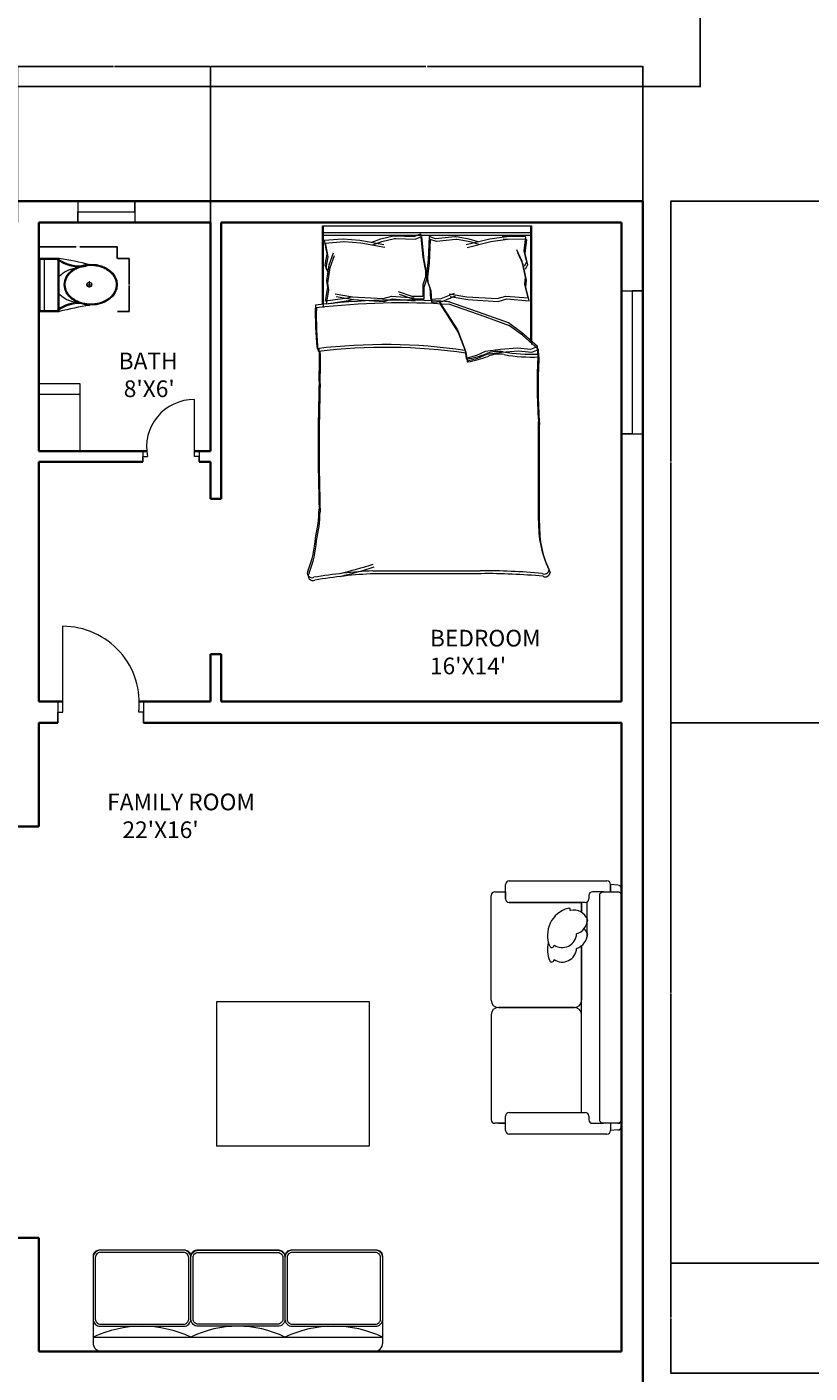
# Model space of a CAD drawing. Units: inches. Extents: x 2185 to 4426, y 1138 to 3073.
# Tile 6 of 14: x 2832 to 3160, y 1834 to 2400. Entities that reach past the tile are written whole.
import ezdxf

# ---------------------------------------------------------------- set-up
doc = ezdxf.new("R2010")
doc.units = ezdxf.units.IN
for name, color, linetype, lineweight in [('A-ANNO-DIMS', 2, 'Continuous', 18), ('A-ANNO-SYMB', 2, 'Continuous', 25), ('A-AREA-IDEN', 7, 'Continuous', 18), ('A-DOOR', 3, 'Continuous', 18), ('A-FLOR-CASE', 32, 'Continuous', 18), ('A-FLOR-FIXT', 9, 'Continuous', 18), ('A-FURN', 8, 'Continuous', 18), ('A-GLAZ', 4, 'Continuous', 18), ('A-WALL', 7, 'Continuous', 35)]:
    doc.layers.add(name, color=color, linetype=linetype, lineweight=lineweight)
doc.styles.get("Standard").update_dxf_attribs({"font": 'arial.ttf'})
doc.dimstyles.get("Standard").update_dxf_attribs({"dimtxt": 0.18, "dimasz": 0.18, "dimexe": 0.18, "dimexo": 0.0625, "dimgap": 0.09, "dimtad": 0, "dimtih": 1, "dimtoh": 1, "dimdec": 4, "dimzin": 0, "dimdsep": 46, "dimtxsty": 'Standard', "dimcen": 0.09, "dimadec": 0, "dimazin": 0, "dimtfac": 1, "dimtdec": 4, "dimtofl": 0, "dimtmove": 0, "dimatfit": 3, "dimfxl": 1, "dimtolj": 1, "dimtzin": 0, "dimarcsym": 0})

# ---------------------------------------------------------------- blocks, each defined once
blk = doc.blocks.new('A$C31115884')
for p, q in [((283, 498), (223, 498)), ((258, 466), (258, 523)), ((0, 200), (0, 0)), ((520, 200), (0, 200)), ((10, 190), (10, 10)), ((510, 190), (10, 190)), ((510, 10), (510, 190)), ((520, 0), (520, 200)), ((510, 54), (0, 54)), ((10, 10), (510, 10)), ((0, 0), (520, 0))]:
    blk.add_line(p, q)
blk.add_circle((256, 496), 23.6)
for centre, radius, start, end in [((2778, -205), 2807, 165.4549, 171.7133), ((-295, 403), 365, 324.2091, 9.3499), ((-295, 403), 375, 324.2091, 9.3499), ((139, 406), 293, 315.8436, 2.6563), ((806, 403), 375, 179.2036, 215.7909), ((806, 403), 365, 170.6501, 215.7909), ((3237, 905), 2807, 188.2867, 194.5451), ((384, 406), 293, 190.2774, 224.1564)]:
    blk.add_arc(centre, radius, start, end)
blk.add_ellipse((256, 510), major_axis=(0, -261), ratio=0.772727)
blk.add_open_spline([(256, 259), (263, 259), (270, 260), (288, 262), (299, 265), (320, 273), (330, 278), (350, 291), (360, 299), (378, 316), (386, 326), (402, 347), (409, 358), (421, 383), (427, 395), (436, 422), (440, 436), (445, 465), (447, 480), (448, 509), (448, 524), (445, 553), (443, 568), (436, 596), (432, 610), (422, 636), (416, 649), (402, 672), (395, 683), (379, 703), (370, 712), (351, 728), (341, 735), (321, 746), (310, 751), (289, 757), (278, 759), (256, 761), (245, 761), (223, 757), (212, 754), (191, 746), (181, 741), (161, 728), (151, 720), (133, 703), (125, 693), (110, 672), (103, 660), (90, 636), (85, 623), (76, 596), (72, 582), (67, 553), (66, 538), (64, 509), (65, 494), (68, 465), (70, 450), (77, 422), (81, 408), (91, 382), (97, 370), (111, 346), (118, 335), (135, 316), (144, 307), (162, 291), (172, 284), (193, 273), (203, 269), (225, 262), (236, 260), (250, 259), (253, 259), (256, 259)], degree=3, knots=[0, 0, 0, 0, 0.110105, 0.110105, 0.285049, 0.285049, 0.459994, 0.459994, 0.634938, 0.634938, 0.809882, 0.809882, 0.984827, 0.984827, 1.159771, 1.159771, 1.334715, 1.334715, 1.50966, 1.50966, 1.684604, 1.684604, 1.859549, 1.859549, 2.034493, 2.034493, 2.209437, 2.209437, 2.384382, 2.384382, 2.559326, 2.559326, 2.73427, 2.73427, 2.909215, 2.909215, 3.084159, 3.084159, 3.259103, 3.259103, 3.434048, 3.434048, 3.608992, 3.608992, 3.783936, 3.783936, 3.958881, 3.958881, 4.133825, 4.133825, 4.30877, 4.30877, 4.483714, 4.483714, 4.658658, 4.658658, 4.833603, 4.833603, 5.008547, 5.008547, 5.183491, 5.183491, 5.358436, 5.358436, 5.53338, 5.53338, 5.708324, 5.708324, 5.883269, 5.883269, 6.058213, 6.058213, 6.233158, 6.233158, 6.283185, 6.283185, 6.283185, 6.283185])
blk = doc.blocks.new('BED-DOUBLE')
for p, q in [((50.74, 96.68), (44.79, 89.9)), ((51.91, 97.09), (45.96, 90.32)), ((53.93, 96.82), (50.74, 96.68, 7.08)), ((51.87, 93.87), (50.74, 96.68)), ((55.1, 97.24), (51.91, 97.09, 7.08)), ((53.04, 94.28), (51.91, 97.09)), ((0, 93.75), (0, 94.16)), ((0, 94.16), (1.36, 94.16)), ((0, 93.75), (48.66, 93.75)), ((0, 6.35), (0, 93.75)), ((1.17, 94.16), (49.83, 94.16)), ((2.8, 6.35), (2.8, 93.75)), ((3.97, 6.77), (3.97, 94.16)), ((4.68, 91.64), (4.5, 81.76)), ((4.68, 91.64), (10.55, 90.94)), ((5.85, 92.05), (5.67, 82.18)), ((5.85, 92.05), (11.72, 91.36)), ((10.55, 90.94), (15.25, 92.03)), ((16.27, 90.59), (11.37, 88.43)), ((11.72, 91.36), (16.42, 92.45)), ((21.63, 91.64), (15.1, 90.17)), ((15.25, 92.03), (17.16, 91.09)), ((22.8, 92.05), (16.27, 90.59)), ((16.42, 92.45), (18.33, 91.51)), ((24.57, 91.29), (21.63, 91.64)), ((25.74, 91.71), (22.8, 92.05)), ((30.31, 92.71), (24.57, 91.29)), ((31.48, 93.13), (25.74, 91.71)), ((29.57, 83.32), (30.31, 92.71)), ((30.74, 83.74), (31.48, 93.13)), ((51.3, 88.2), (51.87, 93.87)), ((52.47, 88.62), (53.04, 94.28)), ((15.1, 90.17), (10.2, 88.01)), ((42, 84.94), (38.32, 74.74)), ((44.79, 89.9), (40.83, 84.52)), ((45.96, 90.32), (42, 84.94)), ((51.87, 81.12), (51.3, 88.2)), ((53.04, 81.54), (52.47, 88.62)), ((4.5, 81.76), (4.65, 83.59)), ((4.65, 83.59), (5.61, 76.65)), ((5.67, 82.18), (5.82, 84.01)), ((5.82, 84.01), (6.78, 77.06)), ((30.59, 79.74), (29.57, 83.32)), ((29.8, 66.92), (30.59, 79.74)), ((31.76, 80.16), (30.74, 83.74)), ((30.97, 67.34), (31.76, 80.16)), ((40.83, 84.52), (37.15, 74.32)), ((52.72, 74.89), (51.87, 81.12)), ((53.89, 75.31), (53.04, 81.54)), ((5.61, 76.65), (8.09, 66.74)), ((6.78, 77.06), (9.26, 67.15)), ((37.15, 74.32), (31.79, 59.08)), ((38.32, 74.74), (32.96, 59.49)), ((54.42, 71.21), (52.72, 74.89)), ((55.59, 71.63), (53.89, 75.31)), ((5.63, 67.91), (4.64, 62.55)), ((6.72, 71.68), (5.63, 67.91)), ((6.8, 68.32), (5.81, 62.97)), ((7.89, 72.1), (6.8, 68.32)), ((55.55, 66.68), (54.42, 71.21)), ((56.72, 67.09), (55.59, 71.63)), ((144.91, 27.55), (144.91, 72.56)), ((146.08, 27.96), (146.08, 72.97)), ((4.64, 62.55), (4.68, 61.96)), ((5.81, 62.97), (5.85, 62.38)), ((5.85, 62.38), (6.62, 54.28)), ((28.58, 59.55), (29.8, 66.92)), ((31.78, 56.65), (29.43, 62.26)), ((29.75, 59.97), (30.97, 67.34)), ((31.79, 55.33), (43.66, 63)), ((32.96, 55.75), (44.83, 63.41)), ((43.66, 63), (51.87, 66.11)), ((44.83, 63.41), (53.04, 66.53)), ((51.87, 66.11), (55.55, 66.68)), ((53.04, 66.53), (56.72, 67.09)), ((4.68, 61.96), (5.45, 53.86)), ((30.61, 56.23), (28.26, 61.85)), ((32.06, 52.16), (31.78, 56.65)), ((5.45, 53.86), (4.56, 51.16)), ((4.56, 51.16), (14.39, 50.71)), ((6.62, 54.28), (5.73, 51.58)), ((5.73, 51.58), (15.56, 51.13)), ((15.56, 51.13), (21.43, 50.44)), ((22.63, 50.17), (26, 51.44)), ((23.8, 50.59), (27.17, 51.86)), ((26, 51.44), (30.89, 51.75)), ((27.17, 51.86), (32.06, 52.16)), ((30.89, 51.75), (30.61, 56.23)), ((3.42, 47.51), (13.2, 48.57)), ((4.48, 44.87), (3.42, 47.51)), ((4.59, 47.93), (14.37, 48.99)), ((5.65, 45.29), (4.59, 47.93)), ((5.38, 37.16), (5.65, 45.29)), ((13.2, 48.57), (19.02, 49.63)), ((14.37, 48.99), (20.19, 50.05)), ((14.39, 50.71), (20.26, 50.02)), ((19.02, 49.63), (21.4, 49.63)), ((20.19, 50.05), (22.57, 50.05)), ((20.26, 50.02), (22.63, 50.17)), ((21.4, 49.63), (24.84, 48.57)), ((21.43, 50.44), (23.8, 50.59)), ((22.57, 50.05), (26.01, 48.99)), ((24.84, 48.57), (29.74, 48.57)), ((26.01, 48.99), (30.91, 48.99)), ((29.74, 48.57), (29.74, 44.08)), ((30.74, 35.86), (31.48, 45.25)), ((30.91, 48.99), (30.91, 44.49)), ((4.21, 36.74), (4.48, 44.87)), ((29.74, 44.08), (27.75, 38.33)), ((30.91, 44.49), (28.91, 38.74)), ((29.57, 35.45), (30.31, 44.83)), ((4.21, 36.15), (4.21, 36.74)), ((5.54, 30.86), (4.21, 36.15)), ((5.38, 36.57), (5.38, 37.16)), ((6.7, 31.28), (5.38, 36.57)), ((30.59, 31.86), (29.57, 35.45)), ((31.76, 32.28), (30.74, 35.86)), ((6.86, 27.16), (5.54, 30.86)), ((6.06, 22.14), (7.92, 32.19)), ((8.03, 27.58), (6.7, 31.28)), ((7.23, 22.56), (9.08, 32.6)), ((29.8, 19.04), (30.59, 31.86)), ((30.97, 19.46), (31.76, 32.28)), ((5.54, 15.15), (6.06, 22.14)), ((6.7, 15.57), (7.23, 22.56)), ((28.58, 11.67), (29.8, 19.04)), ((29.75, 12.09), (30.97, 19.46)), ((29.8, 19.04), (30.39, 16.97)), ((30.39, 16.97), (31.71, 7.65)), ((30.97, 19.46), (31.56, 17.39)), ((31.56, 17.39), (32.88, 8.07)), ((5.5, 14.96), (5.54, 15.15)), ((6.1, 7.13), (5.5, 14.96)), ((6.67, 15.37), (6.7, 15.57)), ((7.27, 7.55), (6.67, 15.37)), ((17.55, 9.65), (12.52, 11.5)), ((1.17, 6.77), (0, 6.77)), ((33.12, 6.35), (0, 6.35)), ((34.29, 6.77), (1.17, 6.77)), ((6.06, 7.12), (11.88, 8.18)), ((7.23, 7.54), (13.05, 8.6)), ((16.38, 9.24), (11.35, 11.09)), ((11.88, 8.18), (16.64, 7.39)), ((13.05, 8.6), (17.81, 7.8)), ((22.99, 8.18), (16.38, 9.24)), ((16.64, 7.39), (18.49, 8.44)), ((24.16, 8.6), (17.55, 9.65)), ((17.81, 7.8), (19.66, 8.86)), ((25.89, 8.71), (22.99, 8.18)), ((27.06, 9.13), (24.16, 8.6)), ((31.71, 7.65), (25.89, 8.71)), ((32.88, 8.07), (27.06, 9.13))]:
    blk.add_line(p, q)
for centre, radius, start, end in [((126.74, 139.68), 42.18, 267.4714, 296.4681), ((145.4, 99.91), 2.02, 332.6588, 86.02), ((-12.17, 93.86), 66.17, 349.8763, 2.5657), ((66.41, 333.3), 236.81, 266.9791, 273.8365), ((-11, 94.28), 66.17, 349.8763, 2.5657), ((67.58, 333.72), 236.81, 266.9791, 273.8365), ((124.02, -8244.93), 8342.06, 90.002168, 90.286887), ((125.19, -8244.52), 8342.06, 90.002168, 90.286887), ((125.57, 139.26), 42.18, 267.4714, 296.4681), ((144.23, 99.5), 2.02, 332.6588, 86.02), ((388.18, 75.25), 243.28, 174.4998, 180.6351), ((389.35, 75.67), 243.28, 174.4998, 180.6351), ((64.12, 79.99), 11.38, 168.6608, 203.7384), ((65.29, 80.41), 11.38, 168.6608, 203.7384), ((2.71, 56.97), 54.23, 10.6617, 19.8806), ((3.88, 57.39), 54.23, 10.6617, 19.8806), ((285.85, 32.47), 235.93, 171.7845, 186.9006), ((287.02, 32.89), 235.93, 171.7845, 186.9006), ((55.66, 66.99), 0.337, 250.2464, 1.1377), ((56.83, 67.41), 0.337, 250.2464, 1.1377), ((332.91, 39.06), 301.67, 176.0865, 186.7821), ((334.08, 39.47), 301.67, 176.0865, 186.7821), ((-43.36, -31.49), 194.68, 13.3832, 17.7053), ((-42.19, -31.08), 194.68, 13.3832, 17.7053), ((367.26, 39.18), 222.65, 182.9958, 189.4091), ((368.43, 39.6), 222.65, 182.9958, 189.4091), ((36.75, 155.73), 152.34, 268.7218, 275.604), ((37.92, 156.15), 152.34, 268.7218, 275.604), ((57.01, -305.95), 311.07, 88.4762, 91.0082), ((58.18, -305.53), 311.07, 88.4762, 91.0082), ((92.56, 886.57), 881.98, 268.22771, 271.71854), ((93.72, 886.99), 881.98, 268.22771, 271.71854), ((117.98, -49.19), 54.19, 76.0648, 88.9113), ((119.15, -48.77), 54.19, 76.0648, 88.9113), ((128.51, -39.61), 43.09, 67.9751, 86.652), ((129.68, -39.19), 43.09, 67.9751, 86.652), ((145.78, 1.99), 1.99, 236.1736, 23.4781), ((146.95, 2.41), 1.99, 236.1736, 23.4781)]:
    blk.add_arc(centre, radius, start, end)
blk = doc.blocks.new('DOOR-SGL-24-ENSUITE')
for p, q in [((21.69, 2.25), (21.69, 26.25)), ((0, 4.5), (0, 0)), ((0, 0), (0, 2.25)), ((0, 2.25), (2, 2.25)), ((23.69, 2.25), (21.69, 2.25)), ((23.69, 4.5), (23.69, 0)), ((23.69, 0), (23.69, 2.25))]:
    blk.add_line(p, q)
blk.add_arc((21.69, 6.17), 20.08, 90, 191.26)
blk = doc.blocks.new('DOOR-SGL-36-BED-E')
for p, q in [((2, 4.5), (2, 40.5)), ((0, 9), (0, 0)), ((35.91, 9), (35.91, 0)), ((0, 0), (0, 4.5)), ((0, 4.5), (2, 4.5)), ((35.91, 4.5), (33.91, 4.5)), ((35.91, 0), (35.91, 4.5))]:
    blk.add_line(p, q)
blk.add_arc((2, 8.36), 32.14, 353.0978, 90)
blk = doc.blocks.new('WIN-PLAN-24IN-01')
for p, q in [((0, 9), (0, 0)), ((24, 4.5), (24, 9)), ((24, 9), (24, 0)), ((0, 0), (0, 4.5)), ((0, 4.5), (0, 4.5)), ((0, 4.5), (24, 4.5))]:
    blk.add_line(p, q)
blk = doc.blocks.new('WIN-PLAN-60IN-03')
for p, q in [((0, 60), (9, 60)), ((9, 60), (4.5, 60)), ((4.5, 60), (4.5, 0)), ((9, 60), (9, 60)), ((4.5, 0), (0, 0)), ((0, 0), (9, 0)), ((9, 0), (9, 0))]:
    blk.add_line(p, q)
blk = doc.blocks.new('BATH-CASEWORK')
for p, q in [((0, 28.5), (17.15, 28.5)), ((17.15, 28.5), (17.15, 0)), ((0, 24), (17.15, 24))]:
    blk.add_line(p, q)
blk = doc.blocks.new('*D48')
at = {"layer": 'A-ANNO-DIMS', "color": 0, "lineweight": -2, "transparency": 16777216}
for p, q in [((2836.52, 2302.3), (2836.52, 2307.35)), ((2836.7, 2307.17), (2852.2, 2307.17)), ((2869.26, 2307.17), (2853.75, 2307.17)), ((2869.44, 2302.3), (2869.44, 2307.35))]:
    blk.add_line(p, q, dxfattribs=at)
at = {"layer": 'A-ANNO-DIMS', "color": 0, "transparency": 16777216}
for points in [[(2836.7, 2307.2), (2836.7, 2307.14), (2836.52, 2307.17)], [(2869.26, 2307.2), (2869.26, 2307.14), (2869.44, 2307.17)]]:
    blk.add_solid(points, dxfattribs=at)
at = {"layer": 'Defpoints', "color": 0, "transparency": 16777216}
for p in [(2869.44, 2307.17), (2836.52, 2302.23), (2869.44, 2302.23)]:
    blk.add_point(p, dxfattribs=at)
at = {"layer": 'A-ANNO-DIMS', "color": 0, "transparency": 16777216, "insert": (2852.98, 2307.17), "char_height": 0.18, "attachment_point": 5}
blk.add_mtext('\\A1;WC 33 TYP.', dxfattribs=at)
blk = doc.blocks.new('*D49')
at = {"layer": 'A-ANNO-DIMS', "color": 0, "lineweight": -2, "transparency": 16777216}
for p, q in [((2869.5, 2302.23), (2874.56, 2302.23)), ((2874.38, 2302.05), (2874.38, 2291.31)), ((2874.38, 2280.2), (2874.38, 2290.95)), ((2869.5, 2280.02), (2874.56, 2280.02))]:
    blk.add_line(p, q, dxfattribs=at)
at = {"layer": 'A-ANNO-DIMS', "color": 0, "transparency": 16777216}
for points in [[(2874.35, 2302.05), (2874.41, 2302.05), (2874.38, 2302.23)], [(2874.35, 2280.2), (2874.41, 2280.2), (2874.38, 2280.02)]]:
    blk.add_solid(points, dxfattribs=at)
at = {"layer": 'Defpoints', "color": 0, "transparency": 16777216}
for p in [(2869.44, 2302.23), (2869.44, 2280.02), (2874.38, 2280.02)]:
    blk.add_point(p, dxfattribs=at)
at = {"layer": 'A-ANNO-DIMS', "color": 0, "transparency": 16777216, "insert": (2874.38, 2291.13), "char_height": 0.18, "attachment_point": 5}
blk.add_mtext('\\A1;22 TYP.', dxfattribs=at)
blk = doc.blocks.new('*D143')
at = {"layer": 'A-ANNO-DIMS', "color": 0, "lineweight": -2, "transparency": 16777216}
for p, q in [((2827.52, 2317.44), (2827.52, 2383.06)), ((2827.7, 2382.88), (2867.82, 2382.88)), ((2908.34, 2382.88), (2868.22, 2382.88)), ((2908.52, 2317.44), (2908.52, 2383.06))]:
    blk.add_line(p, q, dxfattribs=at)
at = {"layer": 'A-ANNO-DIMS', "color": 0, "transparency": 16777216}
for points in [[(2827.7, 2382.91), (2827.7, 2382.85), (2827.52, 2382.88)], [(2908.34, 2382.91), (2908.34, 2382.85), (2908.52, 2382.88)]]:
    blk.add_solid(points, dxfattribs=at)
at = {"layer": 'Defpoints', "color": 0, "transparency": 16777216}
for p in [(2908.52, 2382.88), (2827.52, 2317.38), (2908.52, 2317.38)]:
    blk.add_point(p, dxfattribs=at)
at = {"layer": 'A-ANNO-DIMS', "color": 0, "transparency": 16777216, "insert": (2868.02, 2382.88), "char_height": 0.18, "attachment_point": 5}
blk.add_mtext('\\A1;81', dxfattribs=at)
blk = doc.blocks.new('*D144')
at = {"layer": 'A-ANNO-DIMS', "color": 0, "lineweight": -2, "transparency": 16777216}
for p, q in [((2908.52, 2317.44), (2908.52, 2383.06)), ((2908.7, 2382.88), (2998.88, 2382.88)), ((3089.84, 2382.88), (2999.66, 2382.88)), ((3090.02, 2326.44), (3090.02, 2383.06))]:
    blk.add_line(p, q, dxfattribs=at)
at = {"layer": 'A-ANNO-DIMS', "color": 0, "transparency": 16777216}
for points in [[(2908.7, 2382.91), (2908.7, 2382.85), (2908.52, 2382.88)], [(3089.84, 2382.91), (3089.84, 2382.85), (3090.02, 2382.88)]]:
    blk.add_solid(points, dxfattribs=at)
at = {"layer": 'Defpoints', "color": 0, "transparency": 16777216}
for p in [(3090.02, 2382.88), (3090.02, 2326.38), (2908.52, 2317.38)]:
    blk.add_point(p, dxfattribs=at)
at = {"layer": 'A-ANNO-DIMS', "color": 0, "transparency": 16777216, "insert": (2999.27, 2382.88), "char_height": 0.18, "attachment_point": 5}
blk.add_mtext('\\A1;181.5', dxfattribs=at)
blk = doc.blocks.new('*D152')
at = {"layer": 'A-ANNO-DIMS', "color": 0, "lineweight": -2, "transparency": 16777216}
for p, q in [((3155.01, 1880.56), (3101.64, 1880.56)), ((3101.82, 1880.38), (3101.82, 1857.65)), ((3101.82, 1834.56), (3101.82, 1857.29)), ((3219.79, 1834.38), (3101.64, 1834.38))]:
    blk.add_line(p, q, dxfattribs=at)
at = {"layer": 'A-ANNO-DIMS', "color": 0, "transparency": 16777216}
for points in [[(3101.79, 1880.38), (3101.85, 1880.38), (3101.82, 1880.56)], [(3101.79, 1834.56), (3101.85, 1834.56), (3101.82, 1834.38)]]:
    blk.add_solid(points, dxfattribs=at)
at = {"layer": 'Defpoints', "color": 0, "transparency": 16777216}
for p in [(3101.82, 1880.56), (3155.07, 1880.56), (3219.85, 1834.38)]:
    blk.add_point(p, dxfattribs=at)
at = {"layer": 'A-ANNO-DIMS', "color": 0, "transparency": 16777216, "insert": (3101.82, 1857.47), "char_height": 0.18, "attachment_point": 5}
blk.add_mtext('\\A1;46.19', dxfattribs=at)
blk = doc.blocks.new('*D153')
at = {"layer": 'A-ANNO-DIMS', "color": 0, "lineweight": -2, "transparency": 16777216}
for p, q in [((3219.79, 2107.38), (3101.64, 2107.38)), ((3101.82, 2107.2), (3101.82, 1994.15)), ((3101.82, 1880.74), (3101.82, 1993.79)), ((3155.01, 1880.56), (3101.64, 1880.56))]:
    blk.add_line(p, q, dxfattribs=at)
at = {"layer": 'A-ANNO-DIMS', "color": 0, "transparency": 16777216}
for points in [[(3101.79, 2107.2), (3101.85, 2107.2), (3101.82, 2107.38)], [(3101.79, 1880.74), (3101.85, 1880.74), (3101.82, 1880.56)]]:
    blk.add_solid(points, dxfattribs=at)
at = {"layer": 'Defpoints', "color": 0, "transparency": 16777216}
for p in [(3101.82, 2107.38), (3219.85, 2107.38), (3155.07, 1880.56)]:
    blk.add_point(p, dxfattribs=at)
at = {"layer": 'A-ANNO-DIMS', "color": 0, "transparency": 16777216, "insert": (3101.82, 1993.97), "char_height": 0.18, "attachment_point": 5}
blk.add_mtext('\\A1;226.8', dxfattribs=at)
blk = doc.blocks.new('*D154')
at = {"layer": 'A-ANNO-DIMS', "color": 0, "lineweight": -2, "transparency": 16777216}
for p, q in [((3210.79, 2326.38), (3101.64, 2326.38)), ((3101.82, 2326.2), (3101.82, 2217.06)), ((3101.82, 2107.56), (3101.82, 2216.7)), ((3219.79, 2107.38), (3101.64, 2107.38))]:
    blk.add_line(p, q, dxfattribs=at)
at = {"layer": 'A-ANNO-DIMS', "color": 0, "transparency": 16777216}
for points in [[(3101.79, 2326.2), (3101.85, 2326.2), (3101.82, 2326.38)], [(3101.79, 2107.56), (3101.85, 2107.56), (3101.82, 2107.38)]]:
    blk.add_solid(points, dxfattribs=at)
at = {"layer": 'Defpoints', "color": 0, "transparency": 16777216}
for p in [(3101.82, 2326.38), (3210.85, 2326.38), (3219.85, 2107.38)]:
    blk.add_point(p, dxfattribs=at)
at = {"layer": 'A-ANNO-DIMS', "color": 0, "transparency": 16777216, "insert": (3101.82, 2216.88), "char_height": 0.18, "attachment_point": 5}
blk.add_mtext('\\A1;219', dxfattribs=at)
blk = doc.blocks.new('*D162')
at = {"layer": 'A-ANNO-DIMS', "color": 0, "lineweight": -2, "transparency": 16777216}
for p, q in [((2344.52, 2611.42), (2344.52, 2374.27)), ((3114.02, 2611.42), (3114.02, 2374.27)), ((2344.7, 2374.45), (2728.88, 2374.45)), ((3113.84, 2374.45), (2729.66, 2374.45))]:
    blk.add_line(p, q, dxfattribs=at)
at = {"layer": 'A-ANNO-DIMS', "color": 0, "transparency": 16777216}
for points in [[(2344.7, 2374.48), (2344.7, 2374.42), (2344.52, 2374.45)], [(3113.84, 2374.48), (3113.84, 2374.42), (3114.02, 2374.45)]]:
    blk.add_solid(points, dxfattribs=at)
at = {"layer": 'Defpoints', "color": 0, "transparency": 16777216}
for p in [(2344.52, 2611.48), (3114.02, 2611.48), (3114.02, 2374.45)]:
    blk.add_point(p, dxfattribs=at)
at = {"layer": 'A-ANNO-DIMS', "color": 0, "transparency": 16777216, "insert": (2729.27, 2374.45), "char_height": 0.18, "attachment_point": 5}
blk.add_mtext('\\A1;769.5', dxfattribs=at)

msp = doc.modelspace()

# ---------------------------------------------------------------- linework, layer by layer
at = {"layer": 'A-ANNO-SYMB'}
msp.add_line((3155.074, 1880.563), (4005.21, 1880.563), dxfattribs=at)
at = {"layer": 'A-FURN', "ltscale": 0.03}
for p, q in [((3033.934, 2040.996), (3074.944, 2040.996)), ((3033.934, 2040.996), (3074.944, 2040.996)), ((3026.339, 1990.873), (3026.339, 2034.921)), ((3027.858, 2036.44), (3032.415, 2036.44)), ((3032.415, 2036.44), (3032.415, 2039.477)), ((3032.415, 2036.44), (3032.415, 2039.477)), ((3032.415, 2036.44), (3032.415, 2033.402)), ((3032.415, 2033.402), (3032.415, 2036.44)), ((3067.349, 2034.921), (3067.349, 2033.402)), ((3073.425, 2036.44), (3068.868, 2036.44)), ((3079.5, 2039.234), (3076.463, 2039.477)), ((3076.463, 2039.477), (3076.463, 2036.44)), ((3076.463, 2036.44), (3079.5, 2036.44)), ((3081.019, 2037.715), (3081.019, 1937.955)), ((3081.019, 2034.921), (3081.019, 1940.75)), ((3065.83, 2031.883), (3033.934, 2031.883)), ((3033.934, 2031.883), (3064.312, 2031.883)), ((3064.312, 2027.771), (3064.312, 2031.883)), ((3064.312, 2031.883), (3064.312, 2027.771)), ((3066.598, 2017.209), (3066.598, 2032.091)), ((3064.312, 1943.787), (3064.312, 2013.826)), ((3064.312, 2013.826), (3064.312, 1990.873)), ((3026.339, 1984.797), (3026.339, 1940.75)), ((3061.274, 1987.835), (3029.377, 1987.835)), ((3061.274, 1987.835), (3029.377, 1987.835)), ((3061.274, 1987.835), (3029.377, 1987.835)), ((3029.377, 1987.835), (3061.274, 1987.835)), ((3032.415, 1939.231), (3027.858, 1939.231)), ((3029.377, 1939.231), (3032.415, 1939.231)), ((3032.415, 1939.231), (3032.415, 1942.269)), ((3032.415, 1936.193), (3032.415, 1942.269)), ((3032.415, 1936.193), (3032.415, 1939.231)), ((3033.934, 1943.787), (3065.83, 1943.787)), ((3033.934, 1943.787), (3064.312, 1943.787)), ((3067.349, 1942.269), (3067.349, 1940.75)), ((3068.868, 1939.231), (3073.425, 1939.231)), ((3079.5, 1939.231), (3076.463, 1939.231)), ((3076.463, 1939.231), (3076.463, 1936.193)), ((3076.463, 1939.231), (3076.463, 1936.193)), ((3074.944, 1934.674), (3033.934, 1934.674)), ((3074.944, 1934.674), (3033.934, 1934.674)), ((3079.5, 1936.437), (3076.463, 1936.193))]:
    msp.add_line(p, q, dxfattribs=at)
msp.add_lwpolyline([(3076.463, 2036.44), (3079.5, 2036.44, -0.4142136), (3081.019, 2034.921), (3081.019, 1940.75, -0.4142136), (3079.5, 1939.231), (3073.425, 1939.231, -0.4142136), (3071.906, 1940.75), (3071.906, 2034.921, -0.4142136), (3073.425, 2036.44), (3076.463, 2036.44), (3076.463, 2039.477, 0.4142136), (3074.944, 2040.996)], format="xyb", dxfattribs=at)
at = {"layer": 'A-FURN'}
msp.add_lwpolyline([(2911.192, 1990.398), (2975.098, 1990.398), (2975.098, 1929.574), (2911.192, 1929.574)], close=True, dxfattribs=at)
for points in [[(2859.307, 1882.868), (2859.307, 1857.047, 0.4142136), (2862.345, 1854.009), (2897.28, 1854.009, 0.4142136), (2900.317, 1857.047), (2900.317, 1882.868, 0.4142136), (2897.28, 1885.906), (2862.345, 1885.906, 0.4142136)], [(2860.219, 1882.868), (2860.219, 1857.047, 0.4142136), (2862.345, 1854.921), (2897.28, 1854.921, 0.4142136), (2899.406, 1857.047), (2899.406, 1882.868, 0.4142136), (2897.28, 1884.995), (2862.345, 1884.995, 0.4142136)], [(2939.809, 1882.868), (2939.809, 1857.047, -0.4142136), (2936.771, 1854.009), (2903.355, 1854.009, -0.4142136), (2900.317, 1857.047), (2900.317, 1882.868, -0.4142136), (2903.355, 1885.906), (2936.771, 1885.906, -0.4142136)], [(2938.897, 1882.868), (2938.897, 1857.047, -0.4142136), (2936.771, 1854.921), (2903.355, 1854.921, -0.4142136), (2901.229, 1857.047), (2901.229, 1882.868, -0.4142136), (2903.355, 1884.995), (2936.771, 1884.995, -0.4142136)], [(2939.809, 1882.868), (2939.809, 1857.047, 0.4142136), (2942.846, 1854.009), (2977.781, 1854.009, 0.4142136), (2980.819, 1857.047), (2980.819, 1882.868, 0.4142136), (2977.781, 1885.906), (2942.846, 1885.906, 0.4142136)], [(2940.72, 1882.868), (2940.72, 1857.047, 0.4142136), (2942.846, 1854.921), (2977.781, 1854.921, 0.4142136), (2979.907, 1857.047), (2979.907, 1882.868, 0.4142136), (2977.781, 1884.995), (2942.846, 1884.995, 0.4142136)]]:
    msp.add_lwpolyline(points, format="xyb", close=True, dxfattribs=at)
at = {"layer": 'A-FURN', "ltscale": 0.03}
msp.add_lwpolyline([(2897.857, 1885.906), (2861.738, 1885.906, 0.4142136), (2859.307, 1883.476), (2859.307, 1847.022, 0.4142136), (2862.953, 1843.377), (2977.173, 1843.377, 0.4142136), (2980.819, 1847.022), (2980.819, 1883.476, 0.4142136), (2978.388, 1885.906), (2942.269, 1885.906, 0.4142136), (2939.838, 1883.476, -1), (2939.779, 1883.476, 0.4142136), (2937.348, 1885.906), (2902.778, 1885.906, 0.4142136), (2900.347, 1883.476, -1), (2900.288, 1883.476, 0.4142136)], format="xyb", close=True, dxfattribs=at)
at = {"layer": 'A-FURN'}
msp.add_lwpolyline([(2859.307, 1849.453), (2980.819, 1849.453)], dxfattribs=at)
at = {"layer": 'A-FURN', "ltscale": 0.03}
for centre, radius, start, end in [((3033.934, 2039.477), 1.519, 90, 180), ((3033.934, 2039.477), 1.519, 90, 180), ((3074.944, 2039.477), 1.519, 0, 90), ((3027.858, 2034.921), 1.519, 90, 180), ((3068.868, 2034.921), 1.519, 90, 180), ((3079.5, 2037.715), 1.519, 0, 90), ((3079.5, 2034.921), 1.519, 0, 90), ((3033.934, 2033.402), 1.519, 180, 270), ((3033.934, 2033.402), 1.519, 180, 270), ((3061.735, 2018.147), 11.762, 105.71431, 202.98573), ((3058.906, 2028.836), 0.727, 336.25768, 119.37621), ((3065.83, 2033.402), 1.519, 270, 0), ((3061.014, 2022.469), 6.244, 20.53054, 103.35968), ((3060.035, 2025.256), 6.852, 288.64662, 355.00007), ((3056.147, 2019.081), 6.088, 235.85992, 357.00778), ((3060.035, 2019.18), 6.852, 288.64662, 355.00007), ((3061.014, 2016.393), 6.244, 20.53054, 46.27927), ((3061.735, 2012.072), 11.762, 165.03244, 202.98573), ((3051.769, 2013.982), 0.963, 206.4094, 3.58319), ((3056.147, 2013.005), 6.088, 235.85992, 357.00778), ((3051.769, 2007.907), 0.963, 206.4094, 3.58319), ((3029.377, 1990.873), 3.038, 180, 270), ((3061.274, 1990.873), 3.038, 270, 0), ((3029.377, 1984.797), 3.038, 90, 180), ((3029.377, 1984.797), 3.038, 90, 180), ((3061.274, 1984.797), 3.038, 0, 90), ((3061.274, 1984.797), 3.038, 0, 90), ((3027.858, 1940.75), 1.519, 180, 270), ((3033.934, 1942.269), 1.519, 90, 180), ((3033.934, 1942.269), 1.519, 90, 180), ((3065.83, 1942.269), 1.519, 0, 90), ((3068.868, 1940.75), 1.519, 180, 270), ((3079.5, 1940.75), 1.519, 270, 0), ((3033.934, 1936.193), 1.519, 180, 270), ((3033.934, 1936.193), 1.519, 180, 270), ((3074.944, 1936.193), 1.519, 270, 360), ((3079.5, 1937.955), 1.519, 270, 360)]:
    msp.add_arc(centre, radius, start, end, dxfattribs=at)
at = {"layer": 'A-FURN'}
for centre, radius, start, end in [((2879.812, 1805.658), 48.357, 64.91063, 115.08937), ((2920.063, 1809.202), 44.833, 63.869, 116.131), ((2960.314, 1806.164), 47.899, 64.65382, 115.34618)]:
    msp.add_arc(centre, radius, start, end, dxfattribs=at)
at = {"layer": 'A-WALL'}
for p, q in [((2368.519, 2326.377), (3090.019, 2326.377)), ((3090.019, 2326.377), (3090.019, 1327.377)), ((2836.519, 2317.377), (2836.519, 2221.377)), ((2836.519, 2317.377), (2908.519, 2317.377)), ((2908.519, 2317.377), (2908.519, 2221.377)), ((2913.019, 2317.377), (2913.019, 2201.367)), ((2913.019, 2317.377), (3081.019, 2317.377)), ((3081.019, 2317.377), (3081.019, 2116.377)), ((2836.519, 2221.377), (2881.779, 2221.377)), ((2901.789, 2221.377), (2908.519, 2221.377)), ((2836.519, 2216.877), (2880.096, 2216.877)), ((2836.519, 2216.877), (2836.519, 2116.377)), ((2903.789, 2216.877), (2908.519, 2216.877)), ((2908.519, 2216.877), (2908.519, 2201.367)), ((2908.519, 2201.367), (2913.019, 2201.367)), ((2908.519, 2136.181), (2913.019, 2136.181)), ((2908.519, 2136.181), (2908.519, 2116.377)), ((2913.019, 2136.181), (2913.019, 2116.377)), ((2836.519, 2116.377), (2846.544, 2116.377)), ((2878.676, 2116.377), (2908.519, 2116.377)), ((2913.019, 2116.377), (3081.019, 2116.377)), ((2836.519, 2107.377), (2836.519, 2063.852)), ((2836.519, 2107.377), (2844.544, 2107.377)), ((2880.449, 2107.377), (3081.019, 2107.377)), ((3081.019, 2107.377), (3081.019, 1843.377)), ((2827.519, 2063.852), (2836.519, 2063.852)), ((2827.519, 1891.155), (2836.519, 1891.155)), ((2836.519, 1891.155), (2836.519, 1843.377)), ((2836.519, 1843.377), (3081.019, 1843.377)), ((2836.519, 1843.377), (3081.019, 1843.377))]:
    msp.add_line(p, q, dxfattribs=at)

# ---------------------------------------------------------------- block references
at = {"layer": 'A-DOOR'}
for name, p in [('DOOR-SGL-24-ENSUITE', (2880.096, 2216.877)), ('DOOR-SGL-36-BED-E', (2844.544, 2107.377))]:
    msp.add_blockref(name, p, dxfattribs=at)
at = {"layer": 'A-FLOR-CASE'}
msp.add_blockref('BATH-CASEWORK', (2836.519, 2221.377), dxfattribs=at)
at = {"layer": 'A-FLOR-FIXT', "xscale": 0.0427196977339482, "yscale": 0.0427196977339482, "zscale": 0.0427196977339482, "rotation": 270}
msp.add_blockref('A$C31115884', (2836.519, 2302.234), dxfattribs=at)
at = {"layer": 'A-FURN', "rotation": 270.0000000000002}
msp.add_blockref('BED-DOUBLE', (2949.15, 2316.059), dxfattribs=at)
at = {"layer": 'A-GLAZ'}
for name, p in [('WIN-PLAN-24IN-01', (2852.848, 2317.377)), ('WIN-PLAN-60IN-03', (3081.019, 2228.643))]:
    msp.add_blockref(name, p, dxfattribs=at)

# ---------------------------------------------------------------- texts
at = {"layer": 'A-AREA-IDEN', "char_height": 7, "attachment_point": 1}
for s, width, insert in [("BATH\\P 8'X6'", 209.09036, (2870.016, 2262.774)), ("BEDROOM\\P16'X14'", 298.55411, (3000.645, 2146.404)), ("FAMILY ROOM\\P   22'X16'", 184.53414, (2865.188, 2077.641))]:
    msp.add_mtext_dynamic_manual_height_columns(s, width=width, gutter_width=12.5, heights=[0], dxfattribs=dict(at, insert=insert))

# ---------------------------------------------------------------- dimensions: what is measured, and where the dimension line sits
at = {"layer": 'A-ANNO-DIMS'}
for base, p1, p2, override, picture, middle in [((3114.019, 2374.451), (2344.519, 2611.482), (3114.019, 2611.482), {"dimdec": 1, "dimlfac": 1, "dimrnd": 0, "dimzin": 0, "dimdsep": 46, "dimlunit": 2}, '*D162', (2729.269, 2374.451)), ((2908.519, 2382.877), (2827.519, 2317.377), (2908.519, 2317.377), {"dimdec": 0, "dimlfac": 1, "dimrnd": 0, "dimzin": 0, "dimdsep": 46, "dimlunit": 2}, '*D143', (2868.019, 2382.877)), ((3090.019, 2382.877), (2908.519, 2317.377), (3090.019, 2326.377), {"dimdec": 1, "dimlfac": 1, "dimrnd": 0, "dimzin": 0, "dimdsep": 46, "dimlunit": 2}, '*D144', (2999.269, 2382.877))]:
    dim = msp.add_linear_dim(base=base, p1=p1, p2=p2, dimstyle='Standard', override=override, dxfattribs=at)
    dim.commit()
    dim.dimension.update_dxf_attribs({"geometry": picture, "text_midpoint": middle})
for base, p1, p2, override, picture, middle in [((3101.824, 2326.377), (3219.849, 2107.377), (3210.849, 2326.377), {"dimdec": 0, "dimlfac": 1, "dimrnd": 0, "dimzin": 0, "dimdsep": 46, "dimlunit": 2}, '*D154', (3101.824, 2216.877)), ((3101.824, 2107.377), (3155.074, 1880.563), (3219.849, 2107.377), {"dimdec": 1, "dimlfac": 1, "dimrnd": 0, "dimzin": 0, "dimdsep": 46, "dimlunit": 2}, '*D153', (3101.824, 1993.97)), ((3101.824, 1880.563), (3219.849, 1834.377), (3155.074, 1880.563), {"dimdec": 2, "dimlfac": 1, "dimrnd": 0, "dimzin": 0, "dimdsep": 46, "dimlunit": 2}, '*D152', (3101.824, 1857.47))]:
    dim = msp.add_linear_dim(base=base, p1=p1, p2=p2, angle=90, dimstyle='Standard', override=override, dxfattribs=at)
    dim.commit()
    dim.dimension.update_dxf_attribs({"geometry": picture, "text_midpoint": middle})
dim = msp.add_linear_dim(base=(2869.438, 2307.172), p1=(2836.519, 2302.234), p2=(2869.438, 2302.234), text='WC <> TYP.', dimstyle='Standard', override={"dimdec": 0, "dimlfac": 1, "dimrnd": 0, "dimzin": 0, "dimdsep": 46, "dimlunit": 2}, dxfattribs=at)
dim.commit()
dim.dimension.update_dxf_attribs({"geometry": '*D48', "text_midpoint": (2852.979, 2307.172)})
dim = msp.add_linear_dim(base=(2874.376, 2280.02), p1=(2869.438, 2302.234), p2=(2869.438, 2280.02), angle=270, text='<> TYP.', dimstyle='Standard', override={"dimdec": 0, "dimlfac": 1, "dimrnd": 0, "dimzin": 0, "dimdsep": 46, "dimlunit": 2}, dxfattribs=at)
dim.commit()
dim.dimension.update_dxf_attribs({"geometry": '*D49', "text_midpoint": (2874.376, 2291.127)})

doc.saveas('drawing.dxf')
